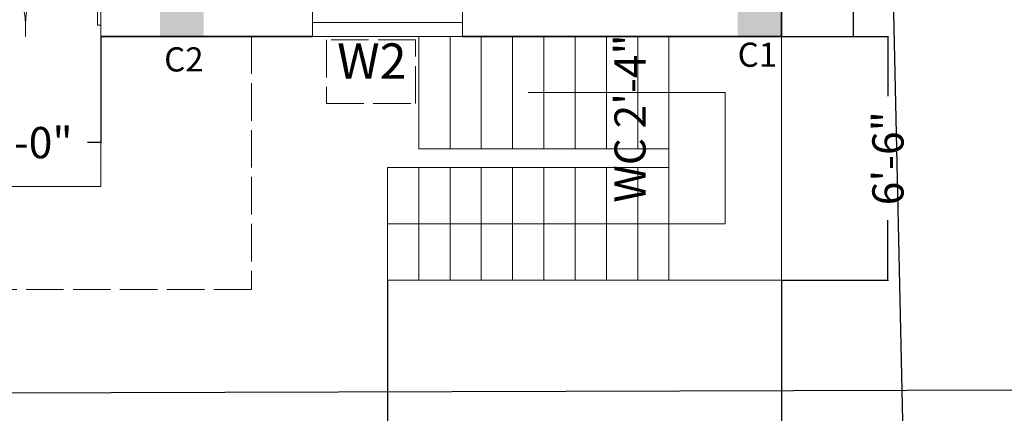
# Model space of a CAD drawing. Units: inches. Extents: x -269 to 4574, y -694 to 313.
# Tile 3 of 19: x 208 to 522, y -486 to -360. Entities that reach past the tile are written whole.
import ezdxf

# ---------------------------------------------------------------- set-up
doc = ezdxf.new("R2010")
doc.units = ezdxf.units.IN
doc.header["$MEASUREMENT"] = 0
doc.linetypes.add('ACAD_ISO02W100', pattern=[15, 12, -3])
for name, color, linetype, lineweight in [('A-ANNO-FRAM', 7, 'ACAD_ISO02W100', 13), ('A-ANNO-IDEN', 6, 'Continuous', 18), ('A-COLS', 5, 'Continuous', 35), ('A-COLS-IDEN', 6, 'Continuous', 18), ('A-ROOF-OVHD', 1, 'ACAD_ISO02W100', 18), ('C-PROP', 7, 'Continuous', 25), ('DIMENSION', 5, 'Continuous', 18), ('DOORS', 3, 'Continuous', 18), ('STAIR', 4, 'Continuous', 20), ('WALL', 1, 'Continuous', 35), ('WINDOWS', 2, 'Continuous', 18)]:
    doc.layers.add(name, color=color, linetype=linetype, lineweight=lineweight)
doc.dimstyles.get("Standard").update_dxf_attribs({"dimtxt": 10, "dimasz": 0.18, "dimexe": 0.18, "dimexo": 0.0625, "dimgap": 0.09, "dimtad": 0, "dimdec": 1, "dimzin": 0, "dimdsep": 46, "dimlunit": 3, "dimtxsty": 'Standard', "dimcen": 0.09, "dimclrt": 7, "dimadec": 0, "dimazin": 0, "dimtfac": 1, "dimtdec": 1, "dimtofl": 0, "dimtmove": 0, "dimatfit": 3, "dimfxl": 1, "dimtolj": 1, "dimtzin": 0, "dimarcsym": 0})

# ---------------------------------------------------------------- blocks, each defined once
blk = doc.blocks.new('*U3')
for p, q in [((0, 0), (0, -6)), ((40, 0), (40, -6))]:
    blk.add_line(p, q)
blk.add_lwpolyline([(0, 0), (0, 40), (1.75, 40), (1.75, 0)], close=True)
blk.add_arc((0, 0), 40, 0, 90)
blk = doc.blocks.new('*D27')
at = {"layer": 'Defpoints', "color": 0, "lineweight": 0, "transparency": 16777216}
for p in [(451.14, 18.27), (451.14, -365.73), (474.13, -365.73)]:
    blk.add_point(p, dxfattribs=at)
at = {"layer": 'DIMENSION', "color": 0, "lineweight": -2, "transparency": 16777216}
for p, q in [((451.2, 18.27), (474.31, 18.27)), ((474.13, 18.09), (474.13, -163.64)), ((474.13, -365.55), (474.13, -183.82)), ((451.2, -365.73), (474.31, -365.73))]:
    blk.add_line(p, q, dxfattribs=at)
at = {"layer": 'DIMENSION', "color": 0, "lineweight": 0, "transparency": 16777216}
for points in [[(474.1, 18.09), (474.16, 18.09), (474.13, 18.27)], [(474.1, -365.55), (474.16, -365.55), (474.13, -365.73)]]:
    blk.add_solid(points, dxfattribs=at)
at = {"layer": 'DIMENSION', "color": 0, "transparency": 16777216, "insert": (474.13, -173.73), "char_height": 10, "attachment_point": 5, "rotation": 90}
blk.add_mtext("\\A1;32'", dxfattribs=at)
blk = doc.blocks.new('*D35')
at = {"layer": 'Defpoints', "color": 0, "lineweight": 0, "transparency": 16777216}
for p in [(478.29, 88), (551.23, -476.8), (527.63, -478.86)]:
    blk.add_point(p, dxfattribs=at)
at = {"layer": 'DIMENSION', "color": 0, "lineweight": -2, "transparency": 16777216}
for p, q in [((478.36, 88.01), (502.07, 90.07)), ((501.91, 89.87), (523.81, -161.74)), ((551.21, -476.62), (529.31, -225.01)), ((527.69, -478.85), (551.41, -476.79))]:
    blk.add_line(p, q, dxfattribs=at)
at = {"layer": 'DIMENSION', "color": 0, "lineweight": 0, "transparency": 16777216}
for points in [[(501.94, 89.88), (501.88, 89.87), (501.89, 90.05)], [(551.24, -476.62), (551.18, -476.63), (551.23, -476.8)]]:
    blk.add_solid(points, dxfattribs=at)
at = {"layer": 'DIMENSION', "color": 0, "transparency": 16777216, "insert": (526.56, -193.38), "char_height": 10, "attachment_point": 5, "rotation": 274.9738}
blk.add_mtext('\\A1;47\'-5.0"', dxfattribs=at)
blk = doc.blocks.new('GLAZ-48IN')
blk.add_line((4.5, 0), (4.5, 48))
blk.add_lwpolyline([(0, 48), (9, 48), (9, 0), (0, 0)], close=True)
blk = doc.blocks.new('COLUMN-9x14-PLAN')
h = blk.add_hatch(color=256)
h.dxf.hatch_style = 1
h.paths.add_polyline_path([(9, 14), (0, 14), (0, 0), (9, 0), (9, 5)])
blk = doc.blocks.new('*D57')
at = {"layer": 'Defpoints', "color": 0, "lineweight": 0, "transparency": 16777216}
for p in [(406.93, -328.51), (402.7, -356.73), (406.93, -356.73)]:
    blk.add_point(p, dxfattribs=at)
at = {"layer": 'DIMENSION', "color": 0, "lineweight": -2, "transparency": 16777216}
for p, q in [((406.87, -328.51), (402.52, -328.51)), ((402.7, -328.69), (402.7, -356.55)), ((406.87, -356.73), (402.52, -356.73)), ((402.7, -356.73), (402.7, -356.91))]:
    blk.add_line(p, q, dxfattribs=at)
at = {"layer": 'DIMENSION', "color": 0, "lineweight": 0, "transparency": 16777216}
for points in [[(402.67, -328.69), (402.73, -328.69), (402.7, -328.51)], [(402.67, -356.55), (402.73, -356.55), (402.7, -356.73)]]:
    blk.add_solid(points, dxfattribs=at)
at = {"layer": 'DIMENSION', "color": 7, "transparency": 16777216, "insert": (402.7, -392), "char_height": 10, "attachment_point": 5, "rotation": 90}
blk.add_mtext('\\A1;WC 2\'-4"', dxfattribs=at)
blk = doc.blocks.new('*D79')
at = {"layer": 'Defpoints', "color": 0, "lineweight": 0, "transparency": 16777216}
for p in [(185.34, -365.73), (233.52, -365.73), (185.34, -399.73)]:
    blk.add_point(p, dxfattribs=at)
at = {"layer": 'DIMENSION', "color": 0, "lineweight": -2, "transparency": 16777216}
for p, q in [((185.34, -365.79), (185.34, -399.91)), ((233.52, -365.79), (233.52, -399.91)), ((185.52, -399.73), (189.58, -399.73)), ((233.34, -399.73), (229.29, -399.73))]:
    blk.add_line(p, q, dxfattribs=at)
at = {"layer": 'DIMENSION', "color": 0, "lineweight": 0, "transparency": 16777216}
for points in [[(185.52, -399.7), (185.52, -399.76), (185.34, -399.73)], [(233.34, -399.7), (233.34, -399.76), (233.52, -399.73)]]:
    blk.add_solid(points, dxfattribs=at)
at = {"layer": 'DIMENSION', "color": 7, "transparency": 16777216, "insert": (209.43, -399.73), "char_height": 10, "attachment_point": 5}
blk.add_mtext('\\A1;4\'-0"', dxfattribs=at)
blk = doc.blocks.new('*D84')
at = {"layer": 'Defpoints', "color": 0, "lineweight": 0, "transparency": 16777216}
for p in [(325.14, -443.73), (451.14, -443.73), (325.14, -540.83)]:
    blk.add_point(p, dxfattribs=at)
at = {"layer": 'DIMENSION', "color": 0, "lineweight": -2, "transparency": 16777216}
for p, q in [((325.14, -443.79), (325.14, -541.01)), ((451.14, -443.79), (451.14, -541.01)), ((325.32, -540.83), (364.48, -540.83)), ((450.96, -540.83), (411.8, -540.83))]:
    blk.add_line(p, q, dxfattribs=at)
at = {"layer": 'DIMENSION', "color": 0, "lineweight": 0, "transparency": 16777216}
for points in [[(325.32, -540.8), (325.32, -540.86), (325.14, -540.83)], [(450.96, -540.8), (450.96, -540.86), (451.14, -540.83)]]:
    blk.add_solid(points, dxfattribs=at)
at = {"layer": 'DIMENSION', "color": 7, "transparency": 16777216, "insert": (388.14, -540.83), "char_height": 10, "attachment_point": 5}
blk.add_mtext('\\A1;10\'-6"', dxfattribs=at)
blk = doc.blocks.new('*D85')
at = {"layer": 'Defpoints', "color": 0, "lineweight": 0, "transparency": 16777216}
for p in [(451.14, -365.73), (451.14, -443.73), (485.14, -443.73)]:
    blk.add_point(p, dxfattribs=at)
at = {"layer": 'DIMENSION', "color": 0, "lineweight": -2, "transparency": 16777216}
for p, q in [((451.2, -365.73), (485.32, -365.73)), ((485.14, -365.91), (485.14, -384.88)), ((485.14, -443.55), (485.14, -424.58)), ((451.2, -443.73), (485.32, -443.73))]:
    blk.add_line(p, q, dxfattribs=at)
at = {"layer": 'DIMENSION', "color": 0, "lineweight": 0, "transparency": 16777216}
for points in [[(485.11, -365.91), (485.17, -365.91), (485.14, -365.73)], [(485.11, -443.55), (485.17, -443.55), (485.14, -443.73)]]:
    blk.add_solid(points, dxfattribs=at)
at = {"layer": 'DIMENSION', "color": 7, "transparency": 16777216, "insert": (485.14, -404.73), "char_height": 10, "attachment_point": 5, "rotation": 90}
blk.add_mtext('\\A1;6\'-6"', dxfattribs=at)

msp = doc.modelspace()

# ---------------------------------------------------------------- linework, layer by layer
at = {"layer": 'A-ANNO-FRAM'}
msp.add_lwpolyline([(334.14, -387.21), (334.14, -366.85), (305.62, -366.85), (305.62, -387.21)], close=True, dxfattribs=at)
at = {"layer": 'A-ROOF-OVHD'}
for p, q in [((281.64, -365.73), (281.64, -446.73)), ((281.64, -446.73), (-40.86, -446.73))]:
    msp.add_line(p, q, dxfattribs=at)
at = {"layer": 'C-PROP'}
for p, q in [((490.29, -506.83), (478.29, 36.26)), ((-68.45, -480.67), (527.63, -478.86))]:
    msp.add_line(p, q, dxfattribs=at)
at = {"layer": 'STAIR'}
for p, q in [((233.52, -365.73), (233.52, -413.73)), ((335.14, -365.73), (335.14, -401.73)), ((345.14, -365.73), (345.14, -401.73)), ((355.14, -365.73), (355.14, -401.73)), ((365.14, -365.73), (365.14, -401.73)), ((375.14, -365.73), (375.14, -401.73)), ((385.14, -365.73), (385.14, -401.73)), ((395.14, -365.73), (395.14, -401.73)), ((405.14, -365.73), (405.14, -401.73)), ((415.14, -365.73), (415.14, -443.73)), ((451.14, -365.73), (451.14, -443.73)), ((370.12, -383.73), (433.14, -383.73)), ((433.14, -425.73), (433.14, -383.73)), ((415.14, -401.73), (335.14, -401.73)), ((415.14, -407.73), (325.14, -407.73)), ((325.14, -407.73), (325.14, -443.73)), ((335.14, -407.73), (335.14, -443.73)), ((345.14, -407.73), (345.14, -443.73)), ((355.14, -407.73), (355.14, -443.73)), ((365.14, -407.73), (365.14, -443.73)), ((375.14, -407.73), (375.14, -443.73)), ((385.14, -407.73), (385.14, -443.73)), ((395.14, -407.73), (395.14, -443.73)), ((405.14, -407.73), (405.14, -443.73)), ((233.52, -413.73), (170.34, -413.73)), ((325.14, -425.73), (433.14, -425.73)), ((451.14, -443.73), (325.14, -443.73))]:
    msp.add_line(p, q, dxfattribs=at)
at = {"layer": 'WALL'}
for p, q in [((451.14, -325.23), (451.14, -365.73)), ((262.14, -365.73), (233.52, -365.73)), ((262.14, -365.73), (301.14, -365.73)), ((451.14, -365.73), (349.14, -365.73))]:
    msp.add_line(p, q, dxfattribs=at)

# ---------------------------------------------------------------- block references
at = {"layer": 'A-COLS', "rotation": 90.0000000000004}
for p in [(266.41, -365.72), (451.14, -365.72)]:
    msp.add_blockref('COLUMN-9x14-PLAN', p, dxfattribs=at)
at = {"layer": 'DOORS', "yscale": 0.6022719637681349, "zscale": 0.6022719637681349}
for p, xscale in [((185.34, -362.13), 0.6022719637681349), ((233.52, -362.13), -0.6022719637681349)]:
    msp.add_blockref('*U3', p, dxfattribs=dict(at, xscale=xscale))
at = {"layer": 'WINDOWS', "extrusion": (0, 0, -1), "zscale": -1, "rotation": 269.9999999999998}
msp.add_blockref('GLAZ-48IN', (-349.14, -356.73), dxfattribs=at)

# ---------------------------------------------------------------- texts
at = {"layer": 'A-ANNO-IDEN'}
msp.add_text('W2', height=11.343, dxfattribs=at).set_placement((309.07, -379.31))
at = {"layer": 'A-COLS-IDEN'}
for s, p in [('C1', (437.1, -375.46)), ('C2', (253.77, -376.96))]:
    msp.add_text(s, height=7.741, dxfattribs=at).set_placement(p)

# ---------------------------------------------------------------- dimensions: what is measured, and where the dimension line sits
at = {"layer": 'DIMENSION'}
dim = msp.add_aligned_dim(p1=(478.29, 88), p2=(527.63, -478.86), distance=23.69, dimstyle='Standard', override={"dimclrd": 0, "dimclre": 0, "dimclrt": 0}, dxfattribs=at)
dim.commit()
dim.dimension.update_dxf_attribs({"geometry": '*D35', "text_midpoint": (526.56, -193.38)})
for base, p1, p2, angle, override, picture, middle in [((474.13, -365.73), (451.14, 18.27), (451.14, -365.73), 90, {"dimclrd": 0, "dimclre": 0, "dimclrt": 0}, '*D27', (474.13, -173.73)), ((185.34, -399.73), (233.52, -365.73), (185.34, -365.73), 180, {"dimdec": 1, "dimlfac": 1, "dimrnd": 0, "dimzin": 1, "dimdsep": 46, "dimlunit": 4, "dimfrac": 2}, '*D79', (209.43, -399.73)), ((485.14, -443.73), (451.14, -365.73), (451.14, -443.73), 270, {"dimdec": 1, "dimlfac": 1, "dimrnd": 0, "dimzin": 1, "dimdsep": 46, "dimlunit": 4, "dimfrac": 2}, '*D85', (485.14, -404.73))]:
    dim = msp.add_linear_dim(base=base, p1=p1, p2=p2, angle=angle, dimstyle='Standard', override=override, dxfattribs=at)
    dim.commit()
    dim.dimension.update_dxf_attribs({"geometry": picture, "text_midpoint": middle})
dim = msp.add_linear_dim(base=(402.7, -356.73), p1=(406.93, -328.51), p2=(406.93, -356.73), angle=270, text='WC <>', dimstyle='Standard', override={"dimdec": 1, "dimlfac": 1, "dimrnd": 0, "dimzin": 1, "dimdsep": 46, "dimlunit": 4, "dimfrac": 2}, dxfattribs=at)
dim.commit()
dim.dimension.update_dxf_attribs({"geometry": '*D57', "text_midpoint": (402.7, -392)})
dim = msp.add_linear_dim(base=(325.14, -540.83), p1=(451.14, -443.73), p2=(325.14, -443.73), dimstyle='Standard', override={"dimdec": 1, "dimlfac": 1, "dimrnd": 0, "dimzin": 1, "dimdsep": 46, "dimlunit": 4, "dimfrac": 2}, dxfattribs=at)
dim.commit()
dim.dimension.update_dxf_attribs({"geometry": '*D84', "text_midpoint": (388.14, -540.83)})

doc.saveas('drawing.dxf')
